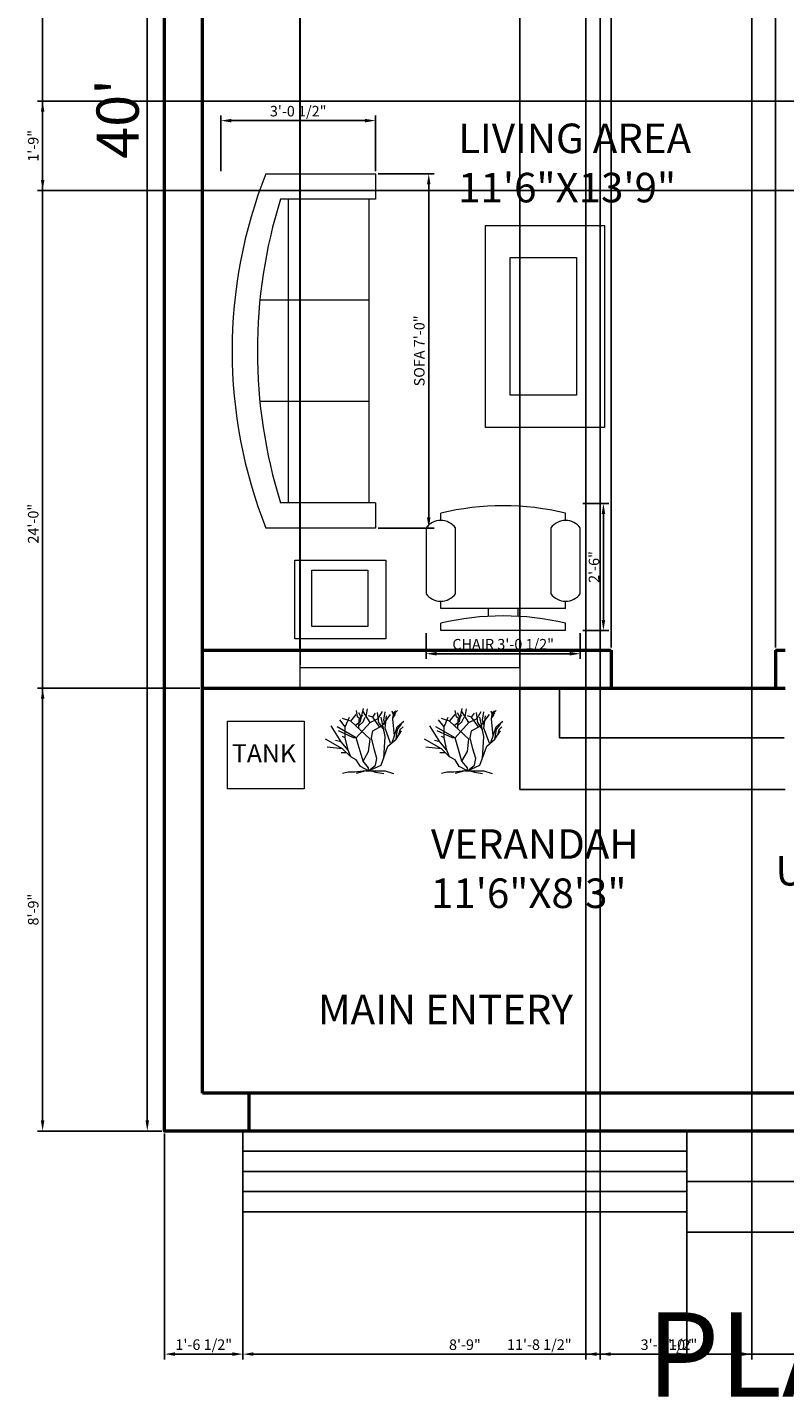
# Model space of a CAD drawing. Units: inches. Extents: x 1854 to 2268, y 1958 to 2535.
# Tile 1 of 4: x 1856 to 2035, y 1958 to 2283. Entities that reach past the tile are written whole.
import ezdxf

# ---------------------------------------------------------------- set-up
doc = ezdxf.new("R2010")
doc.units = ezdxf.units.IN
for name, color, linetype, lineweight in [('A-ANNO-DIMS', 2, 'Continuous', 18), ('A-ANNO-TEXT', 7, 'Continuous', 25), ('A-AREA-IDEN', 7, 'Continuous', 25), ('A-EQPM', 9, 'Continuous', 18), ('A-FLOR-STRS', 7, 'Continuous', 25), ('A-FURN', 8, 'Continuous', 18), ('A-GLAZ', 4, 'Continuous', 18), ('A-WALL', 7, 'Continuous', 50), ('L-PLNT', 94, 'Continuous', 13)]:
    doc.layers.add(name, color=color, linetype=linetype, lineweight=lineweight)
doc.styles.get("Standard").update_dxf_attribs({"font": 'arial.ttf'})
doc.dimstyles.new('ISO-25', dxfattribs={"dimtxt": 2.5, "dimasz": 2.5, "dimexe": 1.25, "dimexo": 0.625, "dimtad": 1, "dimdec": 0, "dimlunit": 3, "dimtxsty": 'Standard', "dimcen": 2.5, "dimadec": 0, "dimazin": 0, "dimtfac": 1, "dimtdec": 0, "dimtmove": 0, "dimatfit": 3, "dimfxl": 1, "dimarcsym": 0})

# ---------------------------------------------------------------- blocks, each defined once
blk = doc.blocks.new('Sofa - Roundback 7 ft.')
for p, q in [((-12.00002, -32.4421), (-12.00003, -6.5971)), ((11.99997, -32.4421), (11.99998, -6.5971)), ((-36.000027, -34), (-36.000027, -11.4696)), ((35.99998, -34), (35.99998, -11.4696)), ((-35.999844, -13.3819), (35.9998, -13.3819)), ((-36.000027, -32.4421), (35.99998, -32.4421))]:
    blk.add_line(p, q)
for points in [[(-36.000027, -34), (-42.000027, -34), (-42.000027, -8)], [(41.99998, -8), (41.99998, -34), (35.99998, -34)]]:
    blk.add_lwpolyline(points)
for centre, radius, start, end in [((0, -114.25), 114.25, 68.43141, 111.5686), ((-0.00001, -127.1968), 121.1968, 72.72033, 107.2797)]:
    blk.add_arc(centre, radius, start, end)
blk = doc.blocks.new('Chair - Desk')
for p, q in [((-8.5, 0), (-8.5, -1)), ((-8.5, 0), (8.5, 0)), ((8.5, 0), (8.5, -1)), ((-8.5, -3), (-8.5, -4)), ((-8.5, -3), (8.5, -3)), ((-2, -3), (-2, -1.9355)), ((2, -1.9576), (2, -3)), ((8.5, -3), (8.5, -4)), ((-10.5, -5), (-10.5, -14)), ((-6.5, -14), (-6.5, -5)), ((6.5, -5), (6.5, -14)), ((10.5, -14), (10.5, -5)), ((-8.5, -15), (-8.5, -16)), ((8.5, -15), (8.5, -16))]:
    blk.add_line(p, q)
for centre, radius, start, end in [((0, 34.625), 36.625, 256.5803, 283.4197), ((-8.5, -6.5), 2.5, 36.8699, 143.1301), ((8.5, -6.5), 2.5, 36.8699, 143.1301), ((-8.5, -12.5), 2.5, 216.8699, 323.1301), ((8.5, -12.5), 2.5, 216.8699, 323.1301), ((0, 19.625), 36.625, 256.5803, 283.4197)]:
    blk.add_arc(centre, radius, start, end)
blk = doc.blocks.new('*U15')
for p, q in [((-14.88, 18.24), (-17.76, 19.2)), ((-16.8, 16.32), (-15.36, 19.68)), ((-14.88, 18.24), (-12.96, 20.64)), ((-12.471, 19.775), (-12.898, 22.044)), ((-11.677, 19.071), (-12.471, 19.775)), ((-11.28, 19.619), (-12.104, 21.184)), ((-11.921, 18.836), (-10.64, 20.401)), ((-11.433, 18.289), (-10.457, 22.749)), ((-10.579, 18.054), (-9.846, 19.697)), ((-8.16, 17.76), (-10.56, 21.6)), ((-9.48, 19.775), (-8.992, 22.592)), ((-7.2, 19.68), (-8.64, 20.16)), ((-8.16, 17.76), (-5.28, 19.2)), ((-7.2, 19.68), (-6.24, 21.12)), ((-4.8, 16.32), (-7.2, 19.68)), ((-5.086, 17.741), (-5.513, 21.34)), ((-5.28, 19.2), (-3.84, 21.6)), ((-2.88, 12.96), (-4.32, 19.68)), ((-3.84, 16.8), (-0.96, 20.64)), ((-3.377, 18.602), (-2.888, 21.575)), ((-2.88, 15.84), (-2.4, 20.16)), ((-0.508, 21.888), (-0.081, 20.558)), ((-0.203, 19.149), (0.102, 21.34)), ((0.346, 13.203), (-0.203, 19.149)), ((-0.142, 19.384), (0.59, 20.401)), ((-0.02, 20.01), (0.896, 21.105)), ((0.041, 20.714), (1.384, 22.044)), ((0.102, 21.34), (0.835, 21.888)), ((-18.24, 11.04), (-21.755, 16.655)), ((-12.96, 12.48), (-19.68, 16.32)), ((-13.92, 12.48), (-19.2, 14.88)), ((-16.8, 16.32), (-18.72, 18.72)), ((-16.8, 12.48), (-16.8, 16.32)), ((-8.16, 12), (-14.88, 18.24)), ((-13.325, 16.724), (-11.433, 18.289)), ((-12.96, 12.48), (-8.16, 17.76)), ((-12.043, 15.628), (-11.921, 18.836)), ((-11.982, 16.802), (-10.579, 18.054)), ((-7.68, 12.48), (-7.2, 14.88)), ((-7.2, 14.88), (-3.84, 16.8)), ((-3.377, 15.315), (-5.086, 17.819)), ((-2.766, 16.802), (-3.377, 18.602)), ((-0.96, 10.56), (-2.88, 15.84)), ((0.346, 13.203), (1.323, 16.254)), ((0.96, 12), (1.44, 15.36)), ((0.96, 12), (2.88, 14.88)), ((1.323, 16.254), (3.642, 18.289)), ((1.44, 15.36), (2.88, 17.28)), ((1.92, 13.44), (2.4, 15.36)), ((2.4, 15.36), (3.36, 16.32)), ((-17.76, 8.64), (-23.663, 11.961)), ((-18.24, 11.04), (-20.16, 11.52)), ((-15.84, 8.16), (-18.24, 11.04)), ((-16.8, 12.48), (-17.76, 12.96)), ((-15.84, 8.16), (-16.8, 12.48)), ((-12.96, 12.48), (-13.92, 12.48)), ((-10.56, 4.32), (-12.96, 12.48)), ((-8.64, 7.68), (-8.16, 12)), ((-6.72, 8.64), (-7.68, 12.48)), ((-4.32, 2.88), (-1.92, 9.6)), ((-3.36, 5.28), (-2.88, 12.96)), ((-1.92, 9.6), (0.96, 12)), ((-0.48, 10.8), (0.346, 13.203)), ((-17.76, 8.64), (-23.128, 9.222)), ((-16.32, 7.2), (-18.24, 7.2)), ((-14.88, 5.76), (-17.76, 8.64)), ((-14.88, 5.76), (-15.84, 8.16)), ((-12.96, 4.8), (-14.88, 5.76)), ((-11.52, 2.4), (-12.96, 4.8)), ((-10.56, 4.32), (-8.64, 7.68)), ((-5.76, 5.28), (-6.72, 8.64)), ((-6.24, 2.88), (-5.76, 5.28)), ((-15.84, 0.48), (-17.76, 0)), ((-13.44, 0.48), (-15.84, 0.48)), ((-9.6, 0.96), (-13.44, 0.48)), ((-9.6, 0.96), (-12.96, 0)), ((-8.64, 0.96), (-11.52, 2.4)), ((-8.64, 1.92), (-10.56, 4.32)), ((-9.6, 0.96), (-7.68, 0.96)), ((-8.64, 0.96), (-4.32, 2.88)), ((-8.64, 0.96), (-6.24, 2.88)), ((-8.64, 0.96), (-8.64, 1.92)), ((-8.64, 0.96), (-2.88, 0.96)), ((-7.68, 0.96), (-6.24, 0.48)), ((-6.24, 0.48), (-3.36, 0)), ((-2.88, 0.96), (0, 0))]:
    blk.add_line(p, q)
blk = doc.blocks.new('*D17')
at = {"layer": 'A-ANNO-DIMS', "color": 0, "lineweight": -2, "transparency": 16777216}
for p, q in [((1887.81, 2500.84), (1883.08, 2500.84)), ((1884.33, 2498.34), (1884.33, 2023.34)), ((1887.81, 2020.84), (1883.08, 2020.84))]:
    blk.add_line(p, q, dxfattribs=at)
at = {"layer": 'A-ANNO-DIMS', "color": 0, "transparency": 16777216}
for points in [[(1883.91, 2498.34), (1884.74, 2498.34), (1884.33, 2500.84)], [(1883.91, 2023.34), (1884.74, 2023.34), (1884.33, 2020.84)]]:
    blk.add_solid(points, dxfattribs=at)
at = {"layer": 'Defpoints', "color": 0, "transparency": 16777216}
for p in [(1888.43, 2500.84), (1884.33, 2020.84), (1888.43, 2020.84)]:
    blk.add_point(p, dxfattribs=at)
at = {"layer": 'A-ANNO-DIMS', "color": 0, "transparency": 16777216, "insert": (1878.6, 2260.84), "char_height": 10, "attachment_point": 5, "rotation": 90}
blk.add_mtext("40'", dxfattribs=at)
blk = doc.blocks.new('*D19')
at = {"layer": 'A-ANNO-DIMS', "color": 0, "lineweight": -2, "transparency": 16777216}
for p, q in [((1939.04, 2247.81), (1952.27, 2247.81)), ((1951.02, 2166.31), (1951.02, 2245.31)), ((1939.04, 2163.81), (1952.27, 2163.81))]:
    blk.add_line(p, q, dxfattribs=at)
at = {"layer": 'A-ANNO-DIMS', "color": 0, "transparency": 16777216}
for points in [[(1950.6, 2245.31), (1951.43, 2245.31), (1951.02, 2247.81)], [(1950.6, 2166.31), (1951.43, 2166.31), (1951.02, 2163.81)]]:
    blk.add_solid(points, dxfattribs=at)
at = {"layer": 'Defpoints', "color": 0, "transparency": 16777216}
for p in [(1938.42, 2247.81), (1951.02, 2247.81), (1938.42, 2163.81)]:
    blk.add_point(p, dxfattribs=at)
at = {"layer": 'A-ANNO-DIMS', "color": 0, "transparency": 16777216, "insert": (1949.1, 2205.81), "char_height": 2.5, "attachment_point": 5, "rotation": 90}
blk.add_mtext('SOFA 7\'-0"', dxfattribs=at)
blk = doc.blocks.new('*D20')
at = {"layer": 'A-ANNO-DIMS', "color": 0, "lineweight": -2, "transparency": 16777216}
for p, q in [((1901.75, 2248.43), (1901.75, 2261.66)), ((1935.92, 2260.41), (1904.25, 2260.41)), ((1938.42, 2248.43), (1938.42, 2261.66))]:
    blk.add_line(p, q, dxfattribs=at)
at = {"layer": 'A-ANNO-DIMS', "color": 0, "transparency": 16777216}
for points in [[(1904.25, 2260.83), (1904.25, 2259.99), (1901.75, 2260.41)], [(1935.92, 2260.83), (1935.92, 2259.99), (1938.42, 2260.41)]]:
    blk.add_solid(points, dxfattribs=at)
at = {"layer": 'Defpoints', "color": 0, "transparency": 16777216}
for p in [(1901.75, 2260.41), (1901.75, 2247.81), (1938.42, 2247.81)]:
    blk.add_point(p, dxfattribs=at)
at = {"layer": 'A-ANNO-DIMS', "color": 0, "transparency": 16777216, "insert": (1920.08, 2262.33), "char_height": 2.5, "attachment_point": 5}
blk.add_mtext('3\'-0 1/2"', dxfattribs=at)
blk = doc.blocks.new('*D21')
at = {"layer": 'A-ANNO-DIMS', "color": 0, "lineweight": -2, "transparency": 16777216}
for p, q in [((1950.37, 2138.87), (1950.37, 2132.76)), ((1986.92, 2138.87), (1986.92, 2132.76)), ((1984.42, 2134.01), (1952.87, 2134.01))]:
    blk.add_line(p, q, dxfattribs=at)
at = {"layer": 'A-ANNO-DIMS', "color": 0, "transparency": 16777216}
for points in [[(1952.87, 2134.42), (1952.87, 2133.59), (1950.37, 2134.01)], [(1984.42, 2134.42), (1984.42, 2133.59), (1986.92, 2134.01)]]:
    blk.add_solid(points, dxfattribs=at)
at = {"layer": 'Defpoints', "color": 0, "transparency": 16777216}
for p in [(1950.37, 2139.49), (1986.92, 2139.49), (1950.37, 2134.01)]:
    blk.add_point(p, dxfattribs=at)
at = {"layer": 'A-ANNO-DIMS', "color": 0, "transparency": 16777216, "insert": (1968.65, 2135.93), "char_height": 2.5, "attachment_point": 5}
blk.add_mtext('CHAIR 3\'-0 1/2"', dxfattribs=at)
blk = doc.blocks.new('*D22')
at = {"layer": 'A-ANNO-DIMS', "color": 0, "lineweight": -2, "transparency": 16777216}
for p, q in [((1987.55, 2169.66), (1993.65, 2169.66)), ((1992.4, 2167.16), (1992.4, 2141.99)), ((1987.55, 2139.49), (1993.65, 2139.49))]:
    blk.add_line(p, q, dxfattribs=at)
at = {"layer": 'A-ANNO-DIMS', "color": 0, "transparency": 16777216}
for points in [[(1991.99, 2167.16), (1992.82, 2167.16), (1992.4, 2169.66)], [(1991.99, 2141.99), (1992.82, 2141.99), (1992.4, 2139.49)]]:
    blk.add_solid(points, dxfattribs=at)
at = {"layer": 'Defpoints', "color": 0, "transparency": 16777216}
for p in [(1986.92, 2169.66), (1986.92, 2139.49), (1992.4, 2139.49)]:
    blk.add_point(p, dxfattribs=at)
at = {"layer": 'A-ANNO-DIMS', "color": 0, "transparency": 16777216, "insert": (1990.5, 2154.57), "char_height": 2.5, "attachment_point": 5, "rotation": 90}
blk.add_mtext('2\'-6"', dxfattribs=at)
blk = doc.blocks.new('*D33')
at = {"layer": 'A-ANNO-DIMS', "color": 0, "lineweight": -2, "transparency": 16777216}
for p, q in [((1991.6, 2440.21), (1991.6, 1966.69)), ((2027.6, 2440.21), (2027.6, 1966.69)), ((1994.1, 1967.94), (2025.1, 1967.94))]:
    blk.add_line(p, q, dxfattribs=at)
at = {"layer": 'A-ANNO-DIMS', "color": 0, "transparency": 16777216}
for points in [[(1994.1, 1968.36), (1994.1, 1967.52), (1991.6, 1967.94)], [(2025.1, 1968.36), (2025.1, 1967.52), (2027.6, 1967.94)]]:
    blk.add_solid(points, dxfattribs=at)
at = {"layer": 'Defpoints', "color": 0, "transparency": 16777216}
for p in [(1991.6, 2440.84), (2027.6, 2440.84), (2027.6, 1967.94)]:
    blk.add_point(p, dxfattribs=at)
at = {"layer": 'A-ANNO-DIMS', "color": 0, "transparency": 16777216, "insert": (2009.6, 1969.84), "char_height": 2.5, "attachment_point": 5}
blk.add_mtext('3\'-0"', dxfattribs=at)
blk = doc.blocks.new('*D35')
at = {"layer": 'A-ANNO-DIMS', "color": 0, "lineweight": -2, "transparency": 16777216}
for p, q in [((1988.27, 2299.21), (1988.27, 1966.69)), ((2027.59, 2299.21), (2027.59, 1966.69)), ((1990.77, 1967.94), (2025.09, 1967.94))]:
    blk.add_line(p, q, dxfattribs=at)
at = {"layer": 'A-ANNO-DIMS', "color": 0, "transparency": 16777216}
for points in [[(1990.77, 1968.36), (1990.77, 1967.52), (1988.27, 1967.94)], [(2025.09, 1968.36), (2025.09, 1967.52), (2027.59, 1967.94)]]:
    blk.add_solid(points, dxfattribs=at)
at = {"layer": 'Defpoints', "color": 0, "transparency": 16777216}
for p in [(1988.27, 2299.84), (2027.59, 2299.84), (2027.59, 1967.94)]:
    blk.add_point(p, dxfattribs=at)
at = {"layer": 'A-ANNO-DIMS', "color": 0, "transparency": 16777216, "insert": (2007.93, 1969.86), "char_height": 2.5, "attachment_point": 5}
blk.add_mtext('3\'-3 1/2"', dxfattribs=at)
blk = doc.blocks.new('*D39')
at = {"layer": 'A-ANNO-DIMS', "color": 0, "lineweight": -2, "transparency": 16777216}
for p, q in [((1920.58, 2131.39), (1920.58, 2530.99)), ((1923.08, 2529.74), (1970.08, 2529.74)), ((1972.58, 2131.39), (1972.58, 2530.99))]:
    blk.add_line(p, q, dxfattribs=at)
at = {"layer": 'A-ANNO-DIMS', "color": 0, "transparency": 16777216}
for points in [[(1923.08, 2530.16), (1923.08, 2529.32), (1920.58, 2529.74)], [(1970.08, 2530.16), (1970.08, 2529.32), (1972.58, 2529.74)]]:
    blk.add_solid(points, dxfattribs=at)
at = {"layer": 'Defpoints', "color": 0, "transparency": 16777216}
for p in [(1972.58, 2529.74), (1920.58, 2130.77), (1972.58, 2130.77)]:
    blk.add_point(p, dxfattribs=at)
at = {"layer": 'A-ANNO-DIMS', "color": 0, "transparency": 16777216, "insert": (1946.58, 2531.61), "char_height": 2.5, "attachment_point": 5}
blk.add_mtext('4\'-4"', dxfattribs=at)
blk = doc.blocks.new('*D40')
at = {"layer": 'A-ANNO-DIMS', "color": 0, "lineweight": -2, "transparency": 16777216}
for p, q in [((1897.43, 2135.46), (1897.43, 2530.99)), ((1899.93, 2529.74), (1917.95, 2529.74)), ((1920.45, 2135.35), (1920.45, 2530.99))]:
    blk.add_line(p, q, dxfattribs=at)
at = {"layer": 'A-ANNO-DIMS', "color": 0, "transparency": 16777216}
for points in [[(1899.93, 2530.16), (1899.93, 2529.32), (1897.43, 2529.74)], [(1917.95, 2530.16), (1917.95, 2529.32), (1920.45, 2529.74)]]:
    blk.add_solid(points, dxfattribs=at)
at = {"layer": 'Defpoints', "color": 0, "transparency": 16777216}
for p in [(1920.45, 2529.74), (1897.43, 2134.84), (1920.45, 2134.72)]:
    blk.add_point(p, dxfattribs=at)
at = {"layer": 'A-ANNO-DIMS', "color": 0, "transparency": 16777216, "insert": (1908.94, 2531.62), "char_height": 2.5, "attachment_point": 5}
blk.add_mtext('1\'-11"', dxfattribs=at)
blk = doc.blocks.new('*D41')
at = {"layer": 'A-ANNO-DIMS', "color": 0, "lineweight": -2, "transparency": 16777216}
for p, q in [((1972.58, 2135.49), (1972.58, 2530.99)), ((1975.08, 2529.74), (1991.71, 2529.74)), ((1994.21, 2135.46), (1994.21, 2530.99))]:
    blk.add_line(p, q, dxfattribs=at)
at = {"layer": 'A-ANNO-DIMS', "color": 0, "transparency": 16777216}
for points in [[(1975.08, 2530.16), (1975.08, 2529.32), (1972.58, 2529.74)], [(1991.71, 2530.16), (1991.71, 2529.32), (1994.21, 2529.74)]]:
    blk.add_solid(points, dxfattribs=at)
at = {"layer": 'Defpoints', "color": 0, "transparency": 16777216}
for p in [(1994.21, 2529.74), (1972.58, 2134.87), (1994.21, 2134.84)]:
    blk.add_point(p, dxfattribs=at)
at = {"layer": 'A-ANNO-DIMS', "color": 0, "transparency": 16777216, "insert": (1983.39, 2531.66), "char_height": 2.5, "attachment_point": 5}
blk.add_mtext('1\'-9 1/2"', dxfattribs=at)
blk = doc.blocks.new('*D42')
at = {"layer": 'A-ANNO-DIMS', "color": 0, "lineweight": -2, "transparency": 16777216}
for p, q in [((1994.21, 2135.46), (1994.21, 2530.99)), ((1996.71, 2529.74), (2030.71, 2529.74)), ((2033.21, 2135.46), (2033.21, 2530.99))]:
    blk.add_line(p, q, dxfattribs=at)
at = {"layer": 'A-ANNO-DIMS', "color": 0, "transparency": 16777216}
for points in [[(1996.71, 2530.16), (1996.71, 2529.32), (1994.21, 2529.74)], [(2030.71, 2530.16), (2030.71, 2529.32), (2033.21, 2529.74)]]:
    blk.add_solid(points, dxfattribs=at)
at = {"layer": 'Defpoints', "color": 0, "transparency": 16777216}
for p in [(2033.21, 2529.74), (1994.21, 2134.84), (2033.21, 2134.84)]:
    blk.add_point(p, dxfattribs=at)
at = {"layer": 'A-ANNO-DIMS', "color": 0, "transparency": 16777216, "insert": (2013.71, 2531.64), "char_height": 2.5, "attachment_point": 5}
blk.add_mtext('3\'-3"', dxfattribs=at)
blk = doc.blocks.new('*D45')
at = {"layer": 'A-ANNO-DIMS', "color": 0, "lineweight": -2, "transparency": 16777216}
for p, q in [((1906.99, 2001.07), (1906.99, 1966.69)), ((2047.43, 1996.21), (2047.43, 1966.69)), ((1909.49, 1967.94), (2044.93, 1967.94))]:
    blk.add_line(p, q, dxfattribs=at)
at = {"layer": 'A-ANNO-DIMS', "color": 0, "transparency": 16777216}
for points in [[(1909.49, 1968.36), (1909.49, 1967.52), (1906.99, 1967.94)], [(2044.93, 1968.36), (2044.93, 1967.52), (2047.43, 1967.94)]]:
    blk.add_solid(points, dxfattribs=at)
at = {"layer": 'Defpoints', "color": 0, "transparency": 16777216}
for p in [(1906.99, 2001.7), (2047.43, 1996.84), (2047.43, 1967.94)]:
    blk.add_point(p, dxfattribs=at)
at = {"layer": 'A-ANNO-DIMS', "color": 0, "transparency": 16777216, "insert": (1977.21, 1969.86), "char_height": 2.5, "attachment_point": 5}
blk.add_mtext('11\'-8 1/2"', dxfattribs=at)
blk = doc.blocks.new('*D49')
at = {"layer": 'A-ANNO-DIMS', "color": 0, "lineweight": -2, "transparency": 16777216}
for p, q in [((1888.43, 2020.21), (1888.43, 1966.69)), ((1906.99, 2020.21), (1906.99, 1966.69)), ((1890.93, 1967.94), (1904.49, 1967.94))]:
    blk.add_line(p, q, dxfattribs=at)
at = {"layer": 'A-ANNO-DIMS', "color": 0, "transparency": 16777216}
for points in [[(1890.93, 1968.36), (1890.93, 1967.52), (1888.43, 1967.94)], [(1904.49, 1968.36), (1904.49, 1967.52), (1906.99, 1967.94)]]:
    blk.add_solid(points, dxfattribs=at)
at = {"layer": 'Defpoints', "color": 0, "transparency": 16777216}
for p in [(1888.43, 2020.84), (1906.99, 2020.84), (1906.99, 1967.94)]:
    blk.add_point(p, dxfattribs=at)
at = {"layer": 'A-ANNO-DIMS', "color": 0, "transparency": 16777216, "insert": (1897.71, 1969.86), "char_height": 2.5, "attachment_point": 5}
blk.add_mtext('1\'-6 1/2"', dxfattribs=at)
blk = doc.blocks.new('*D59')
at = {"layer": 'A-ANNO-DIMS', "color": 0, "lineweight": -2, "transparency": 16777216}
for p, q in [((2098.61, 2265.03), (1858.28, 2265.03)), ((1859.53, 2246.34), (1859.53, 2262.53)), ((2098.32, 2243.84), (1858.28, 2243.84))]:
    blk.add_line(p, q, dxfattribs=at)
at = {"layer": 'A-ANNO-DIMS', "color": 0, "transparency": 16777216}
for points in [[(1859.12, 2262.53), (1859.95, 2262.53), (1859.53, 2265.03)], [(1859.12, 2246.34), (1859.95, 2246.34), (1859.53, 2243.84)]]:
    blk.add_solid(points, dxfattribs=at)
at = {"layer": 'Defpoints', "color": 0, "transparency": 16777216}
for p in [(1859.53, 2265.03), (2099.24, 2265.03), (2098.94, 2243.84)]:
    blk.add_point(p, dxfattribs=at)
at = {"layer": 'A-ANNO-DIMS', "color": 0, "transparency": 16777216, "insert": (1857.63, 2254.43), "char_height": 2.5, "attachment_point": 5, "rotation": 90}
blk.add_mtext('1\'-9"', dxfattribs=at)
blk = doc.blocks.new('*D67')
at = {"layer": 'A-ANNO-DIMS', "color": 0, "lineweight": -2, "transparency": 16777216}
for p, q in [((1896.81, 2125.84), (1858.28, 2125.84)), ((1859.53, 2023.34), (1859.53, 2123.34)), ((1887.81, 2020.84), (1858.28, 2020.84))]:
    blk.add_line(p, q, dxfattribs=at)
at = {"layer": 'A-ANNO-DIMS', "color": 0, "transparency": 16777216}
for points in [[(1859.12, 2123.34), (1859.95, 2123.34), (1859.53, 2125.84)], [(1859.12, 2023.34), (1859.95, 2023.34), (1859.53, 2020.84)]]:
    blk.add_solid(points, dxfattribs=at)
at = {"layer": 'Defpoints', "color": 0, "transparency": 16777216}
for p in [(1859.53, 2125.84), (1897.43, 2125.84), (1888.43, 2020.84)]:
    blk.add_point(p, dxfattribs=at)
at = {"layer": 'A-ANNO-DIMS', "color": 0, "transparency": 16777216, "insert": (1857.63, 2073.34), "char_height": 2.5, "attachment_point": 5, "rotation": 90}
blk.add_mtext('8\'-9"', dxfattribs=at)
blk = doc.blocks.new('*D68')
at = {"layer": 'A-ANNO-DIMS', "color": 0, "lineweight": -2, "transparency": 16777216}
for p, q in [((1896.81, 2308.84), (1858.28, 2308.84)), ((1859.53, 2023.34), (1859.53, 2306.34)), ((1887.81, 2020.84), (1858.28, 2020.84))]:
    blk.add_line(p, q, dxfattribs=at)
at = {"layer": 'A-ANNO-DIMS', "color": 0, "transparency": 16777216}
for points in [[(1859.12, 2306.34), (1859.95, 2306.34), (1859.53, 2308.84)], [(1859.12, 2023.34), (1859.95, 2023.34), (1859.53, 2020.84)]]:
    blk.add_solid(points, dxfattribs=at)
at = {"layer": 'Defpoints', "color": 0, "transparency": 16777216}
for p in [(1859.53, 2308.84), (1897.43, 2308.84), (1888.43, 2020.84)]:
    blk.add_point(p, dxfattribs=at)
at = {"layer": 'A-ANNO-DIMS', "color": 0, "transparency": 16777216, "insert": (1857.63, 2164.84), "char_height": 2.5, "attachment_point": 5, "rotation": 90}
blk.add_mtext('24\'-0"', dxfattribs=at)
blk = doc.blocks.new('*D78')
at = {"layer": 'A-ANNO-DIMS', "color": 0, "lineweight": -2, "transparency": 16777216}
for p, q in [((1906.99, 2001.07), (1906.99, 1966.69)), ((2012.17, 2001.07), (2012.17, 1966.69)), ((1909.49, 1967.94), (2009.67, 1967.94))]:
    blk.add_line(p, q, dxfattribs=at)
at = {"layer": 'A-ANNO-DIMS', "color": 0, "transparency": 16777216}
for points in [[(1909.49, 1968.36), (1909.49, 1967.52), (1906.99, 1967.94)], [(2009.67, 1968.36), (2009.67, 1967.52), (2012.17, 1967.94)]]:
    blk.add_solid(points, dxfattribs=at)
at = {"layer": 'Defpoints', "color": 0, "transparency": 16777216}
for p in [(1906.99, 2001.7), (2012.17, 2001.7), (2012.17, 1967.94)]:
    blk.add_point(p, dxfattribs=at)
at = {"layer": 'A-ANNO-DIMS', "color": 0, "transparency": 16777216, "insert": (1959.58, 1969.84), "char_height": 2.5, "attachment_point": 5}
blk.add_mtext('8\'-9"', dxfattribs=at)

msp = doc.modelspace()

# ---------------------------------------------------------------- linework, layer by layer
at = {"layer": 'A-EQPM'}
msp.add_lwpolyline([(1903.3, 2118.01), (1921.49, 2118.01), (1921.49, 2102.01), (1903.3, 2102.01)], close=True, dxfattribs=at)
at = {"layer": 'A-FLOR-STRS'}
for p, q in [((1972.6, 2126.01), (1972.6, 2101.79)), ((1981.99, 2125.79), (1981.99, 2114.06)), ((1981.99, 2114.06), (2035.22, 2114.06)), ((1972.6, 2101.79), (2035.43, 2101.79)), ((1906.99, 2020.84), (1906.99, 2001.7)), ((1906.99, 2020.84), (2012.17, 2020.84)), ((2012.17, 1996.84), (2012.17, 2020.84)), ((2012.17, 2020.84), (2047.43, 2020.84)), ((1906.99, 2016.05), (2012.17, 2016.05)), ((1906.99, 2011.27), (2012.17, 2011.27)), ((1906.99, 2006.48), (2012.17, 2006.48)), ((2012.17, 2008.84), (2047.43, 2008.84)), ((1906.99, 2001.7), (2012.17, 2001.7)), ((2012.17, 1996.84), (2047.43, 1996.84))]:
    msp.add_line(p, q, dxfattribs=at)
at = {"layer": 'A-FURN'}
for points in [[(1964.49, 2235.56), (1992.65, 2235.56), (1992.65, 2187.62), (1964.49, 2187.62)], [(1970.33, 2227.94), (1985.99, 2227.94), (1985.99, 2195.34), (1970.33, 2195.34)], [(1919.3, 2156.2), (1940.84, 2156.2), (1940.84, 2137.56), (1919.3, 2137.56)], [(1923.33, 2153.85), (1936.58, 2153.85), (1936.58, 2140.45), (1923.33, 2140.45)]]:
    msp.add_lwpolyline(points, close=True, dxfattribs=at)
at = {"layer": 'A-GLAZ'}
for p, q in [((1920.45, 2134.72), (1920.45, 2125.89)), ((1972.58, 2130.77), (1972.58, 2134.87)), ((1972.58, 2134.87), (1972.58, 2125.82)), ((1920.58, 2130.77), (1972.58, 2130.77))]:
    msp.add_line(p, q, dxfattribs=at)
at = {"layer": 'A-WALL'}
for p, q in [((1897.43, 2029.84), (1897.43, 2440.84)), ((1897.43, 2134.84), (1994.21, 2134.84)), ((1994.21, 2134.85), (1994.21, 2125.94)), ((2033.21, 2134.85), (2033.21, 2125.94)), ((2033.21, 2134.84), (2035.43, 2134.84)), ((1897.43, 2125.84), (2035.43, 2125.84)), ((2179.43, 2029.84), (1897.43, 2029.84)), ((1908.42, 2029.84), (1908.42, 2020.84))]:
    msp.add_line(p, q, dxfattribs=at)
msp.add_lwpolyline([(1888.43, 2500.84), (2188.43, 2500.84), (2188.43, 2020.84), (1888.43, 2020.84)], close=True, dxfattribs=at)

# ---------------------------------------------------------------- block references
at = {"layer": 'A-FURN', "rotation": 90}
msp.add_blockref('Sofa - Roundback 7 ft.', (1904.42, 2205.81), dxfattribs=at)
at = {"layer": 'A-FURN', "xscale": 1.740485294342291, "yscale": 1.740485294342291, "zscale": 1.740485294342291, "rotation": 180}
msp.add_blockref('Chair - Desk', (1968.65, 2139.49), dxfattribs=at)
at = {"layer": 'L-PLNT', "xscale": 0.6787869852083795, "yscale": 0.6787869852083795, "zscale": 0.6787869852083795}
for p in [(1942.64, 2105.61), (1966.06, 2105.61)]:
    msp.add_blockref('*U15', p, dxfattribs=at)

# ---------------------------------------------------------------- texts
at = {"layer": 'A-ANNO-TEXT', "attachment_point": 1}
for s, width, gutter_width, insert, char_height in [('TANK', 46.9871, 7.72, (1904.38, 2112.55), 4.325), ('UP', 76.0498, 12.5, (2033.17, 2086.06), 7), ('MAIN ENTERY', 76.0498, 12.5, (1924.75, 2053.15), 7), ('PLAN', 76.0498, 12.5, (2002.62, 1977.86), 20)]:
    msp.add_mtext_dynamic_manual_height_columns(s, width=width, gutter_width=gutter_width, heights=[0], dxfattribs=dict(at, insert=insert, char_height=char_height))
at = {"layer": 'A-AREA-IDEN', "char_height": 7, "attachment_point": 1}
for s, insert in [('LIVING AREA\\P11\'6"X13\'9"', (1957.98, 2259.7)), ('VERANDAH\\P11\'6"X8\'3"', (1951.54, 2092.38))]:
    msp.add_mtext_dynamic_manual_height_columns(s, width=76.0498, gutter_width=12.5, heights=[0], dxfattribs=dict(at, insert=insert))

# ---------------------------------------------------------------- dimensions: what is measured, and where the dimension line sits
at = {"layer": 'A-ANNO-DIMS'}
for base, p1, p2, picture, middle in [((1920.45, 2529.74), (1897.43, 2134.84), (1920.45, 2134.72), '*D40', (1908.94, 2531.62)), ((1972.58, 2529.74), (1920.58, 2130.77), (1972.58, 2130.77), '*D39', (1946.58, 2531.61)), ((1994.21, 2529.74), (1972.58, 2134.87), (1994.21, 2134.84), '*D41', (1983.39, 2531.66)), ((2033.21, 2529.74), (1994.21, 2134.84), (2033.21, 2134.84), '*D42', (2013.71, 2531.64)), ((2027.6, 1967.94), (1991.6, 2440.84), (2027.6, 2440.84), '*D33', (2009.6, 1969.84)), ((2027.59, 1967.94), (1988.27, 2299.84), (2027.59, 2299.84), '*D35', (2007.93, 1969.86)), ((1906.99, 1967.94), (1888.43, 2020.84), (1906.99, 2020.84), '*D49', (1897.71, 1969.86)), ((2047.43, 1967.94), (1906.99, 2001.7), (2047.43, 1996.84), '*D45', (1977.21, 1969.86)), ((2012.17, 1967.94), (1906.99, 2001.7), (2012.17, 2001.7), '*D78', (1959.58, 1969.84))]:
    dim = msp.add_linear_dim(base=base, p1=p1, p2=p2, dimstyle='ISO-25', override={"dimdec": 1, "dimlfac": 1, "dimrnd": 0, "dimzin": 1, "dimdsep": 46, "dimlunit": 4, "dimfrac": 2}, dxfattribs=at)
    dim.commit()
    dim.dimension.update_dxf_attribs({"geometry": picture, "text_midpoint": middle})
for base, p1, p2, angle, override, picture, middle in [((1884.33, 2020.84), (1888.43, 2500.84), (1888.43, 2020.84), 90, {"dimtxt": 10, "dimclrd": 0, "dimclre": 0, "dimclrt": 0}, '*D17', (1878.6, 2260.84)), ((1859.53, 2308.84), (1888.43, 2020.84), (1897.43, 2308.84), 90, {"dimdec": 1, "dimlfac": 1, "dimrnd": 0, "dimzin": 1, "dimdsep": 46, "dimlunit": 4, "dimfrac": 2}, '*D68', (1857.63, 2164.84)), ((1859.53, 2265.03), (2098.94, 2243.84), (2099.24, 2265.03), 90, {"dimdec": 1, "dimlfac": 1, "dimrnd": 0, "dimzin": 1, "dimdsep": 46, "dimlunit": 4, "dimfrac": 2}, '*D59', (1857.63, 2254.43)), ((1901.75, 2260.41), (1938.42, 2247.81), (1901.75, 2247.81), 180, {"dimdec": 1, "dimlfac": 1, "dimrnd": 0, "dimzin": 1, "dimdsep": 46, "dimlunit": 4, "dimfrac": 2}, '*D20', (1920.08, 2262.33)), ((1992.4, 2139.49), (1986.92, 2169.66), (1986.92, 2139.49), 270, {"dimdec": 1, "dimlfac": 1, "dimrnd": 0, "dimzin": 1, "dimdsep": 46, "dimlunit": 4, "dimfrac": 2}, '*D22', (1990.5, 2154.57)), ((1859.53, 2125.84), (1888.43, 2020.84), (1897.43, 2125.84), 90, {"dimdec": 1, "dimlfac": 1, "dimrnd": 0, "dimzin": 1, "dimdsep": 46, "dimlunit": 4, "dimfrac": 2}, '*D67', (1857.63, 2073.34))]:
    dim = msp.add_linear_dim(base=base, p1=p1, p2=p2, angle=angle, dimstyle='ISO-25', override=override, dxfattribs=at)
    dim.commit()
    dim.dimension.update_dxf_attribs({"geometry": picture, "text_midpoint": middle})
for base, p1, p2, angle, text, picture, middle in [((1951.02, 2247.81), (1938.42, 2163.81), (1938.42, 2247.81), 90, 'SOFA <>', '*D19', (1949.1, 2205.81)), ((1950.3707, 2134.0079), (1986.9209, 2139.4905), (1950.3707, 2139.4905), 180, 'CHAIR <>', '*D21', (1968.6458, 2135.9264))]:
    dim = msp.add_linear_dim(base=base, p1=p1, p2=p2, angle=angle, text=text, dimstyle='ISO-25', override={"dimdec": 1, "dimlfac": 1, "dimrnd": 0, "dimzin": 1, "dimdsep": 46, "dimlunit": 4, "dimfrac": 2}, dxfattribs=at)
    dim.commit()
    dim.dimension.update_dxf_attribs({"geometry": picture, "text_midpoint": middle})

doc.saveas('drawing.dxf')
